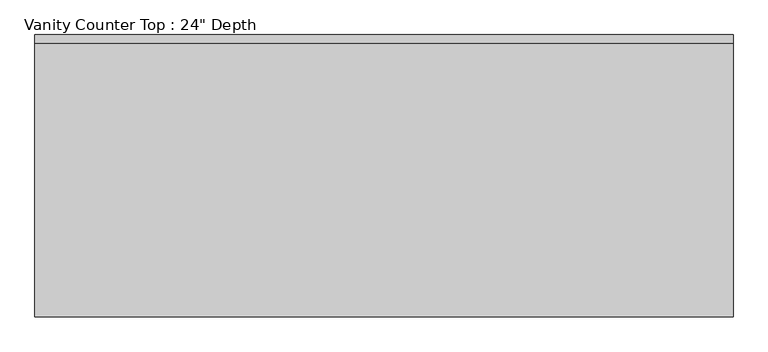
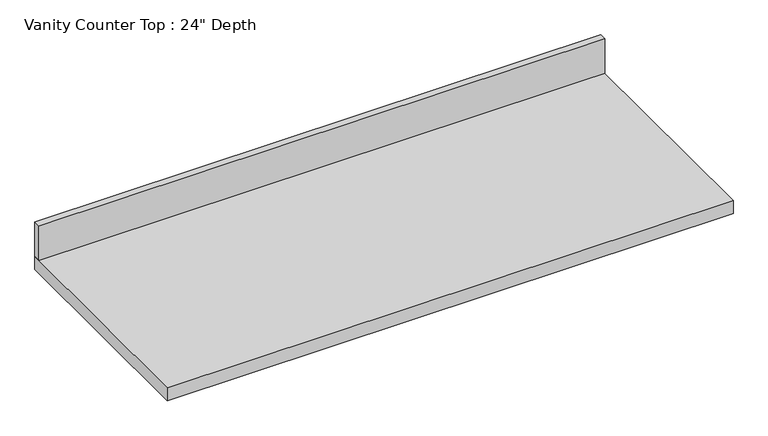
"""IFC4 building model written with IfcOpenShell, lengths in millimetres: furniture geometry."""

from ifc_helpers import new_model, si_unit, frame, origin, place, context, project, spatial, polyline, outline, extrude, source, transform, mapped, element, save


def furniture_49332987(model_context):
    return source(origin(), model_context, "Body", "SweptSolid", [
        extrude(outline(polyline([(369.1437228, 0.0), (369.1437228, -635.0), (-1200.4622951, -635.0), (-1200.4622951, 0.0), (369.1437228, 0.0)])), frame((0.0, 0.0, 749.3), z_axis=(0.0, 0.0, 1.0), x_axis=(1.0, 0.0, 0.0)), (0.0, 0.0, 1.0), 38.1),
        extrude(outline(polyline([(-1200.4622951, 0.0), (369.1437228, 0.0), (369.1437228, -19.05), (-1200.4622951, -19.05), (-1200.4622951, 0.0)])), frame((0.0, 0.0, 787.4), z_axis=(0.0, 0.0, 1.0), x_axis=(1.0, 0.0, 0.0)), (0.0, 0.0, 1.0), 101.6),
    ])


if __name__ == "__main__":
    model = new_model("IFC4")
    model_context = context("Model", 3, world=origin())
    ifc_project = project(units=[si_unit("LENGTHUNIT", "METRE", prefix="MILLI")], contexts=[model_context])
    site = spatial("IfcSite", under=ifc_project)
    building = spatial("IfcBuilding", under=site)
    placement = place(None, origin())
    furniture_shape = furniture_49332987(model_context)
    element("IfcFurniture", 1, ObjectType="Vanity Counter Top : 24\" Depth", at=placement, inside=building, context=model_context, shape_type="MappedRepresentation", body=[
        mapped(furniture_shape, transform((0.0, 0.0, 0.0), x_axis=(1.0, 0.0, 0.0), y_axis=(0.0, 1.0, 0.0), z_axis=(0.0, 0.0, 1.0))),
    ])
    save(model, "model.ifc")

# Revit data of these elements
# Type "Vanity Counter Top : 24\" Depth"
#   Counter Thickness = 0' - 1 1/2"
#   Depth = 2' - 1"
#   Height = 2' - 7"
#   Length [instance default] = 4' - 0"
#   Counter Top Material = Counter Top
#   Default Elevation = 0
# Element 1 (IfcFurniture, "Vanity Counter Top : 24\" Depth")
#   Length = 5' - 1.79551"
#   Materials on its faces: "Counter Top"
# Materials
#   "Counter Top": colour RGB 226 177 128, transparency 0
